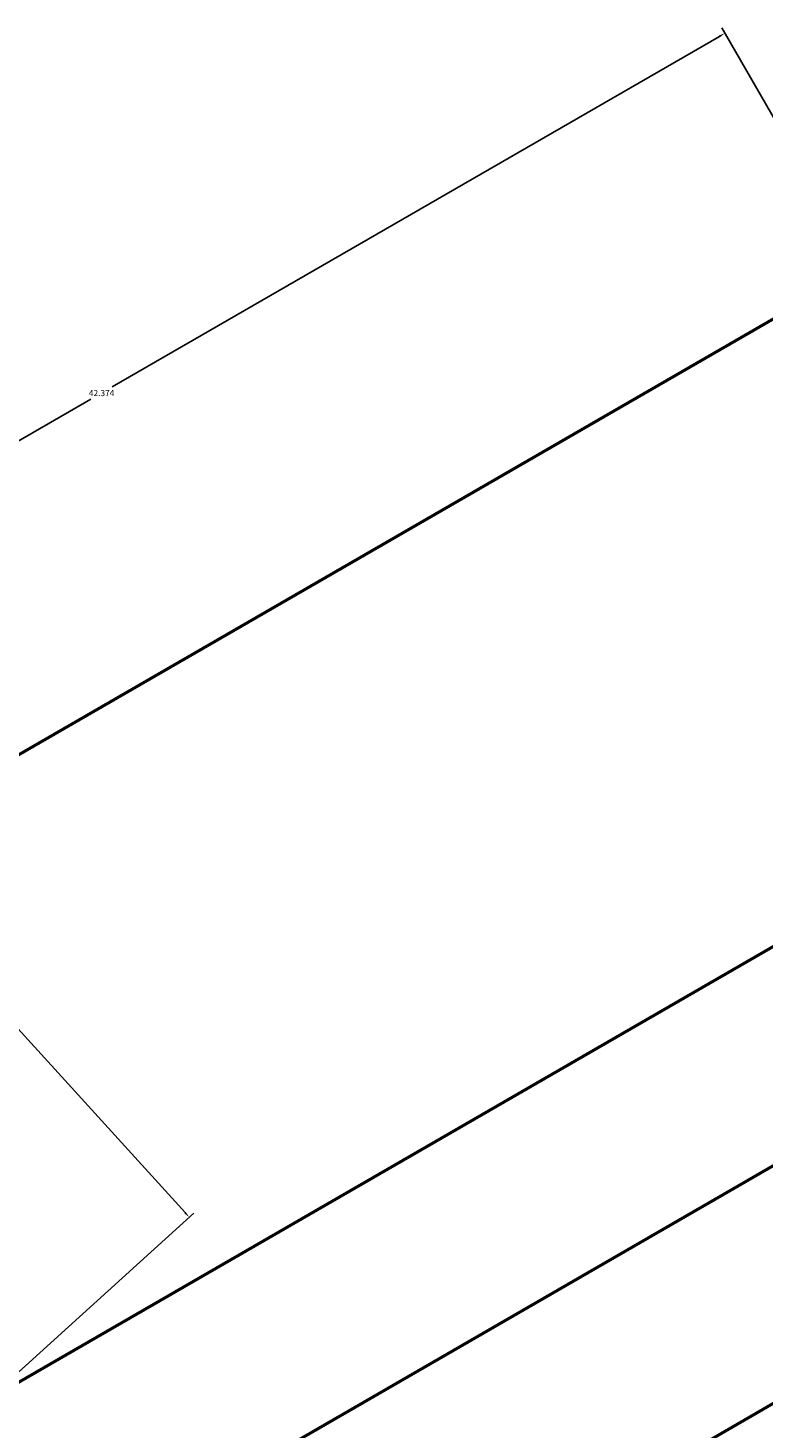
# Model space of a CAD drawing. Units: millimetres. Extents: x 2919 to 3075, y 2801 to 2951.
# Tile 8 of 14: x 2963 to 2984, y 2910 to 2951. Entities that reach past the tile are written whole.
import ezdxf

# ---------------------------------------------------------------- set-up
doc = ezdxf.new("R2010")
doc.units = ezdxf.units.MM
doc.layers.add('M-DIMS', color=2, linetype='Continuous', lineweight=18)
doc.layers.add('M-OUTL', color=7, linetype='Continuous', lineweight=50)
doc.styles.get("Standard").update_dxf_attribs({"font": 'arial.ttf'})
doc.dimstyles.get("Standard").update_dxf_attribs({"dimtxt": 0.18, "dimasz": 0.18, "dimexe": 0.18, "dimexo": 0.0625, "dimgap": 0.09, "dimtad": 0, "dimtih": 1, "dimtoh": 1, "dimdec": 4, "dimzin": 0, "dimdsep": 46, "dimtxsty": 'Standard', "dimcen": 0.09, "dimadec": 0, "dimazin": 0, "dimtfac": 1, "dimtdec": 4, "dimtofl": 0, "dimtmove": 0, "dimatfit": 3, "dimfxl": 1, "dimtolj": 1, "dimtzin": 0, "dimarcsym": 0})

# ---------------------------------------------------------------- blocks, each defined once
blk = doc.blocks.new('*D16')
at = {"layer": 'Defpoints', "color": 0, "transparency": 16777216}
for p in [(2983.323, 2951.131), (2987.323, 2944.203), (2950.626, 2923.015)]:
    blk.add_point(p, dxfattribs=at)
at = {"layer": 'M-DIMS', "color": 0, "lineweight": -2, "transparency": 16777216}
for p, q in [((2987.292, 2944.257), (2983.233, 2951.287)), ((2983.167, 2951.041), (2965.29, 2940.719)), ((2946.782, 2930.034), (2964.659, 2940.355)), ((2950.595, 2923.07), (2946.536, 2930.1))]:
    blk.add_line(p, q, dxfattribs=at)
at = {"layer": 'M-DIMS', "color": 0, "transparency": 16777216}
for points in [[(2983.152, 2951.067), (2983.182, 2951.015), (2983.323, 2951.131)], [(2946.767, 2930.06), (2946.797, 2930.008), (2946.626, 2929.944)]]:
    blk.add_solid(points, dxfattribs=at)
at = {"layer": 'M-DIMS', "color": 0, "transparency": 16777216, "insert": (2964.975, 2940.537), "char_height": 0.18, "attachment_point": 5}
blk.add_mtext('\\A1;42.374', dxfattribs=at)
blk = doc.blocks.new('*D22')
at = {"layer": 'Defpoints', "color": 0, "transparency": 16777216}
for p in [(2950.626, 2923.015), (2967.553, 2916.27), (2961.63, 2910.893)]:
    blk.add_point(p, dxfattribs=at)
at = {"layer": 'M-DIMS', "color": 0, "lineweight": -2, "transparency": 16777216}
for p, q in [((2950.672, 2923.057), (2956.683, 2928.513)), ((2956.67, 2928.259), (2961.886, 2922.513)), ((2967.432, 2916.404), (2962.216, 2922.149)), ((2961.676, 2910.935), (2967.686, 2916.391))]:
    blk.add_line(p, q, dxfattribs=at)
at = {"layer": 'M-DIMS', "color": 0, "transparency": 16777216}
for points in [[(2956.693, 2928.279), (2956.648, 2928.239), (2956.549, 2928.392)], [(2967.454, 2916.424), (2967.41, 2916.383), (2967.553, 2916.27)]]:
    blk.add_solid(points, dxfattribs=at)
at = {"layer": 'M-DIMS', "color": 0, "transparency": 16777216, "insert": (2962.051, 2922.331), "char_height": 0.18, "attachment_point": 5}
blk.add_mtext('\\A1;16.37', dxfattribs=at)

msp = doc.modelspace()

# ---------------------------------------------------------------- linework, layer by layer
at = {"layer": 'M-OUTL'}
for p, q in [((2960.6821, 2903.8932), (2995.3232, 2923.8932)), ((2966.7443, 2900.3932), (3001.3853, 2920.3932))]:
    msp.add_line(p, q, dxfattribs=at)
for points in [[(2928.6099, 2892.1931), (2950.6258, 2923.0154), (2987.3232, 2944.2026)], [(2941.6296, 2882.8932), (2961.6296, 2910.8932), (2995.3232, 2930.3462)], [(2941.6296, 2882.8932), (2961.6296, 2910.8932), (2995.3232, 2930.3462)]]:
    msp.add_lwpolyline(points, dxfattribs=at)

# ---------------------------------------------------------------- dimensions: what is measured, and where the dimension line sits
at = {"layer": 'M-DIMS'}
for base, p2, angle, override, picture, middle in [((2983.3232, 2951.1308), (2987.3232, 2944.2026), 30, {"dimdec": 3, "dimlfac": 1, "dimrnd": 0, "dimzin": 0, "dimdsep": 46, "dimlunit": 2}, '*D16', (2964.9745, 2940.5372)), ((2967.5531, 2916.2702), (2961.6296, 2910.8932), 312.23116, {"dimdec": 2, "dimlfac": 1, "dimrnd": 0, "dimzin": 0, "dimdsep": 46, "dimlunit": 2}, '*D22', (2962.0512, 2922.3313))]:
    dim = msp.add_linear_dim(base=base, p1=(2950.6258, 2923.0154), p2=p2, angle=angle, dimstyle='Standard', override=override, dxfattribs=at)
    dim.commit()
    dim.dimension.update_dxf_attribs({"geometry": picture, "text_midpoint": middle})

doc.saveas('drawing.dxf')
